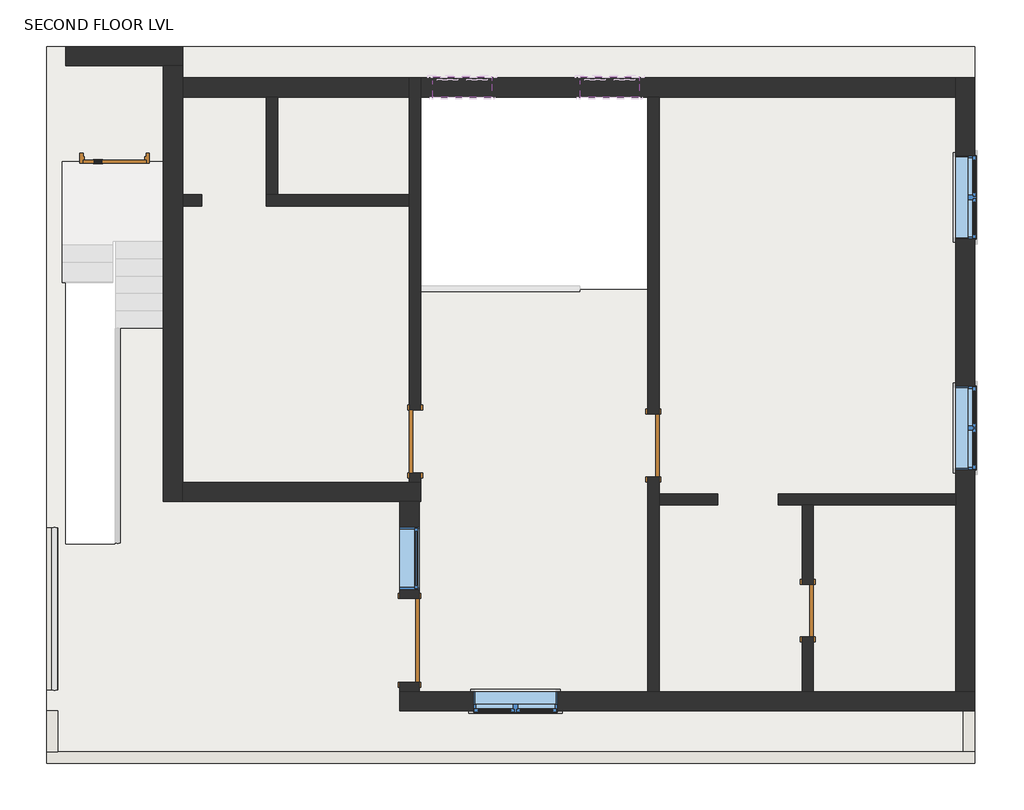
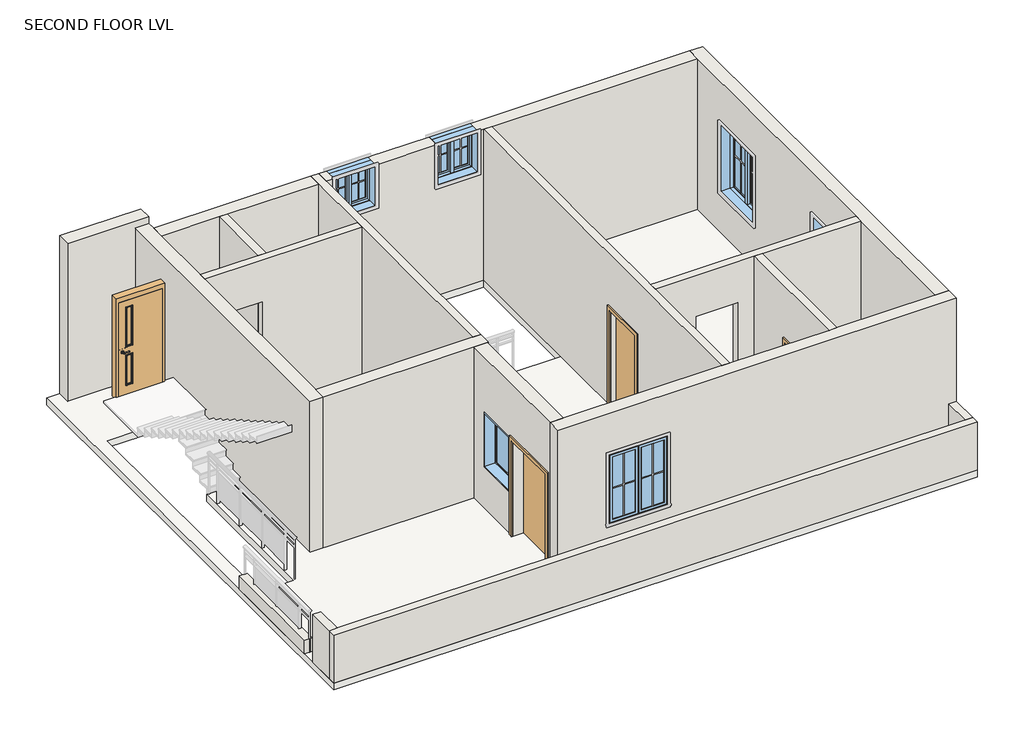
# One storey, part 1 of 2: 18 walls, 6 windows, 5 doors, 1 slab.
"""IFC4 building model written with IfcOpenShell, lengths in millimetres."""

from ifc_helpers import new_model, si_unit, frame, origin, place, context, project, spatial, polyline, outline, extrude, faceted_brep, transform, mapped, element, save
from components import door_52fb15b9, door_3dc6c820, door_d2d7de5b, door_44a3b16d, door_21b9160b, window_60f40170, window_6eb120d7, window_49c71971

model = new_model("IFC4")

# Units and contexts
model_context = context("Model", 3, world=origin())
ifc_project = project(units=[si_unit("LENGTHUNIT", "METRE", prefix="MILLI")], contexts=[model_context])

# Site, building, storey
site = spatial("IfcSite", under=ifc_project)
building = spatial("IfcBuilding", under=site)
storey = spatial("IfcBuildingStorey", under=building, Name="SECOND FLOOR LVL", Elevation=7010.4)

# Doors
placement = place(None, origin())
door_shape = door_52fb15b9(model_context)
element("IfcDoor", 1, ObjectType="Door-Passage-Single-Vision_Two_Lite : 36\" x 84\"", at=placement, inside=storey, context=model_context, shape_type="MappedRepresentation", body=[
    mapped(door_shape, transform((-6092.5155596, 7334.5576853, 7835.9), x_axis=(1.0, 0.0, 0.0), y_axis=(0.0, 1.0, 0.0), z_axis=(0.0, 0.0, 1.0))),
])
door_2_shape = door_3dc6c820(model_context)
element("IfcDoor", 2, ObjectType="Single-Flush : 30\" x 84\"", at=placement, inside=storey, context=model_context, shape_type="MappedRepresentation", body=[
    mapped(door_2_shape, transform((3997.6344404, 698.8076853, 7010.4), x_axis=(0.0, 1.0, 0.0), y_axis=(-1.0, 0.0, 0.0), z_axis=(0.0, 0.0, 1.0))),
])
door_3_shape = door_d2d7de5b(model_context)
element("IfcDoor", 3, ObjectType="Single-Flush : 36\" x 84\"", at=placement, inside=storey, context=model_context, shape_type="MappedRepresentation", body=[
    mapped(door_3_shape, transform((1749.7344404, 3105.4576853, 7010.4), x_axis=(0.0, -1.0, 0.0), y_axis=(1.0, 0.0, 0.0), z_axis=(0.0, 0.0, 1.0))),
])
door_4_shape = door_44a3b16d(model_context)
element("IfcDoor", 4, ObjectType="Single-Flush : 36\" x 84\"", at=placement, inside=storey, context=model_context, shape_type="MappedRepresentation", body=[
    mapped(door_4_shape, transform((-1717.3655596, 3162.6076853, 7010.4), x_axis=(0.0, -1.0, 0.0), y_axis=(1.0, 0.0, 0.0), z_axis=(0.0, 0.0, 1.0))),
])
door_5_shape = door_21b9160b(model_context)
element("IfcDoor", 5, ObjectType="Single-Flush : 48\" x 84\"", at=placement, inside=storey, context=model_context, shape_type="MappedRepresentation", body=[
    mapped(door_5_shape, transform((-1799.9155596, 267.0076853, 7010.4), x_axis=(0.0, -1.0, 0.0), y_axis=(1.0, 0.0, 0.0), z_axis=(0.0, 0.0, 1.0))),
])

# Slab
element("IfcSlab", 6, ObjectType="Generic - 6\"", at=placement, inside=storey, context=model_context, shape_type="SweptSolid", body=[
    extrude(outline(polyline([(6429.6844404, 8915.7076853), (6429.6844404, -1523.6923147), (-7083.1155596, -1523.6923147), (-7083.1155596, 8915.7076853), (6429.6844404, 8915.7076853)]), holes=[polyline([(-6092.5155596, 1670.3576853), (-6092.5155596, 4813.6076853), (-5381.3155596, 4813.6076853), (-5381.3155596, 7188.5076853), (-6092.5155596, 7188.5076853), (-6803.7155596, 7188.5076853), (-6803.7155596, 1670.3576853), (-6092.5155596, 1670.3576853)]), polyline([(1667.1844404, 8179.1076853), (-1634.8155596, 8179.1076853), (-1634.8155596, 5385.1076853), (-555.3155596, 5385.1076853), (1667.1844404, 5385.1076853), (1667.1844404, 8179.1076853)])]), frame((0.0, 0.0, 6858.0), z_axis=(0.0, 0.0, 1.0), x_axis=(1.0, 0.0, 0.0)), (0.0, 0.0, 1.0), 152.4),
])

# Walls
element("IfcWall", 7, ObjectType="4", at=placement, inside=storey, context=model_context, shape_type="Brep", body=[
    faceted_brep([(-1799.9155596, 2705.4076853, 9144.0), (-1799.9155596, 2705.4076853, 7010.4), (-1799.9155596, 2565.7076853, 7010.4), (-1799.9155596, 2565.7076853, 10363.2), (-1799.9155596, 5181.9076853, 10363.2), (-1799.9155596, 5410.5076853, 10363.2), (-1799.9155596, 6591.6076853, 10363.2), (-1799.9155596, 6756.7076853, 10363.2), (-1799.9155596, 8179.1076853, 10363.2), (-1799.9155596, 8458.5076853, 10363.2), (-1799.9155596, 8458.5076853, 7010.4), (-1799.9155596, 8179.1076853, 7010.4), (-1799.9155596, 6756.7076853, 7010.4), (-1799.9155596, 6591.6076853, 7010.4), (-1799.9155596, 3619.8076853, 7010.4), (-1799.9155596, 3619.8076853, 9144.0), (-1634.8155596, 2565.7076853, 7010.4), (-1634.8155596, 2705.4076853, 7010.4), (-1634.8155596, 2705.4076853, 9144.0), (-1634.8155596, 3619.8076853, 9144.0), (-1634.8155596, 3619.8076853, 7010.4), (-1634.8155596, 8179.1076853, 7010.4), (-1634.8155596, 8458.5076853, 7010.4), (-1634.8155596, 8458.5076853, 10363.2), (-1634.8155596, 8179.1076853, 10363.2), (-1634.8155596, 2565.7076853, 10363.2)], [[[0, 1, 2, 3, 4, 5, 6, 7, 8, 9, 10, 11, 12, 13, 14, 15]], [[16, 17, 18, 19, 20, 21, 22, 23, 24, 25]], [[2, 1, 17, 16]], [[14, 13, 12, 11, 10, 22, 21, 20]], [[9, 8, 7, 6, 5, 4, 3, 25, 24, 23]], [[3, 2, 16, 25]], [[18, 17, 1, 0]], [[19, 18, 0, 15]], [[20, 19, 15, 14]], [[10, 9, 23, 22]]]),
])
element("IfcWall", 8, ObjectType="4", at=placement, inside=storey, context=model_context, shape_type="Brep", body=[
    faceted_brep([(1667.1844404, 2648.2576853, 9144.0), (1667.1844404, 2648.2576853, 7010.4), (1667.1844404, -482.2923147, 7010.4), (1667.1844404, -482.2923147, 10363.2), (1667.1844404, 8179.1076853, 10363.2), (1667.1844404, 8179.1076853, 7010.4), (1667.1844404, 3562.6576853, 7010.4), (1667.1844404, 3562.6576853, 9144.0), (1832.2844404, -482.2923147, 7010.4), (1832.2844404, 2235.5076853, 7010.4), (1832.2844404, 2400.6076853, 7010.4), (1832.2844404, 2648.2576853, 7010.4), (1832.2844404, 2648.2576853, 9144.0), (1832.2844404, 3562.6576853, 9144.0), (1832.2844404, 3562.6576853, 7010.4), (1832.2844404, 8179.1076853, 7010.4), (1832.2844404, 8179.1076853, 10363.2), (1832.2844404, 5410.5076853, 10363.2), (1832.2844404, 5181.9076853, 10363.2), (1832.2844404, 2514.9076853, 10363.2), (1832.2844404, 2400.6076853, 10363.2), (1832.2844404, 2235.5076853, 10363.2), (1832.2844404, -482.2923147, 10363.2)], [[[0, 1, 2, 3, 4, 5, 6, 7]], [[8, 9, 10, 11, 12, 13, 14, 15, 16, 17, 18, 19, 20, 21, 22]], [[6, 5, 15, 14]], [[2, 1, 11, 10, 9, 8]], [[4, 3, 22, 21, 20, 19, 18, 17, 16]], [[3, 2, 8, 22]], [[5, 4, 16, 15]], [[12, 11, 1, 0]], [[13, 12, 0, 7]], [[14, 13, 7, 6]]]),
])
element("IfcWall", 9, ObjectType="4", at=placement, inside=storey, context=model_context, shape_type="SweptSolid", body=[
    extrude(outline(polyline([(2235.5076853, 7010.4), (1079.8076853, 7010.4), (1079.8076853, 9144.0), (317.8076853, 9144.0), (317.8076853, 7010.4), (-482.2923147, 7010.4), (-482.2923147, 10363.2), (2235.5076853, 10363.2), (2235.5076853, 7010.4)])), frame((3915.0844404, 0.0, 0.0), z_axis=(1.0, 0.0, 0.0), x_axis=(0.0, 1.0, 0.0)), (0.0, 0.0, 1.0), 165.1),
])
element("IfcWall", 10, ObjectType="4", at=placement, inside=storey, context=model_context, shape_type="Brep", body=[
    faceted_brep([(6150.2844404, 2235.5076853, 7010.4), (6150.2844404, 2235.5076853, 10363.2), (4080.1844404, 2235.5076853, 10363.2), (3915.0844404, 2235.5076853, 10363.2), (1832.2844404, 2235.5076853, 10363.2), (1832.2844404, 2235.5076853, 7010.4), (2687.0502939, 2235.5076853, 7010.4), (2687.0502939, 2235.5076853, 9448.8), (3567.6284806, 2235.5076853, 9448.8), (3567.6284806, 2235.5076853, 7010.4), (3915.0844404, 2235.5076853, 7010.4), (4080.1844404, 2235.5076853, 7010.4), (6150.2844404, 2400.6076853, 10363.2), (6150.2844404, 2400.6076853, 7010.4), (3567.6284806, 2400.6076853, 7010.4), (3567.6284806, 2400.6076853, 9448.8), (2687.0502939, 2400.6076853, 9448.8), (2687.0502939, 2400.6076853, 7010.4), (1832.2844404, 2400.6076853, 7010.4), (1832.2844404, 2400.6076853, 10363.2), (2022.7844404, 2400.6076853, 10363.2), (5307.0165832, 2400.6076853, 10363.2), (5611.8165832, 2400.6076853, 10363.2)], [[[0, 1, 2, 3, 4, 5, 6, 7, 8, 9, 10, 11]], [[12, 13, 14, 15, 16, 17, 18, 19, 20, 21, 22]], [[5, 18, 17, 6]], [[13, 0, 11, 10, 9, 14]], [[4, 3, 2, 1, 12, 22, 21, 20, 19]], [[1, 0, 13, 12]], [[5, 4, 19, 18]], [[7, 16, 15, 8]], [[16, 7, 6, 17]], [[8, 15, 14, 9]]]),
])
element("IfcWall", 11, ObjectType="4", at=placement, inside=storey, context=model_context, shape_type="SweptSolid", body=[
    extrude(outline(polyline([(-3882.7155596, 6756.7076853), (-3882.7155596, 8179.1076853), (-3717.6155596, 8179.1076853), (-3717.6155596, 6756.7076853), (-3882.7155596, 6756.7076853)])), frame((0.0, 0.0, 7010.4), z_axis=(0.0, 0.0, 1.0), x_axis=(1.0, 0.0, 0.0)), (0.0, 0.0, 1.0), 3352.8),
])
element("IfcWall", 12, ObjectType="4", at=placement, inside=storey, context=model_context, shape_type="Brep", body=[
    faceted_brep([(-1799.9155596, 6591.6076853, 7010.4), (-1799.9155596, 6591.6076853, 10363.2), (-5101.9155596, 6591.6076853, 10363.2), (-5101.9155596, 6591.6076853, 7010.4), (-4820.8679217, 6591.6076853, 7010.4), (-4820.8679217, 6591.6076853, 9448.8), (-3885.4711324, 6591.6076853, 9448.8), (-3885.4711324, 6591.6076853, 7010.4), (-1799.9155596, 6756.7076853, 10363.2), (-1799.9155596, 6756.7076853, 7010.4), (-3717.6155596, 6756.7076853, 7010.4), (-3882.7155596, 6756.7076853, 7010.4), (-3885.4711324, 6756.7076853, 7010.4), (-3885.4711324, 6756.7076853, 9448.8), (-4820.8679217, 6756.7076853, 9448.8), (-4820.8679217, 6756.7076853, 7010.4), (-5101.9155596, 6756.7076853, 7010.4), (-5101.9155596, 6756.7076853, 10363.2), (-3882.7155596, 6756.7076853, 10363.2), (-3717.6155596, 6756.7076853, 10363.2)], [[[0, 1, 2, 3, 4, 5, 6, 7]], [[8, 9, 10, 11, 12, 13, 14, 15, 16, 17, 18, 19]], [[9, 0, 7, 12, 11, 10]], [[3, 16, 15, 4]], [[2, 1, 8, 19, 18, 17]], [[1, 0, 9, 8]], [[3, 2, 17, 16]], [[5, 14, 13, 6]], [[14, 5, 4, 15]], [[6, 13, 12, 7]]]),
])
element("IfcWall", 13, ObjectType="4", at=placement, inside=storey, context=model_context, shape_type="SweptSolid", body=[
    extrude(outline(polyline([(-6918.0155596, 1905.3076853), (-6918.0155596, -456.8923147), (-7083.1155596, -456.8923147), (-7083.1155596, 1905.3076853), (-6918.0155596, 1905.3076853)])), frame((0.0, 0.0, 7010.4), z_axis=(0.0, 0.0, 1.0), x_axis=(1.0, 0.0, 0.0)), (0.0, 0.0, 1.0), 304.8),
])
element("IfcWall", 14, ObjectType="4", at=placement, inside=storey, context=model_context, shape_type="Brep", body=[
    faceted_brep([(6429.6844404, -1358.5923147, 7010.4), (6264.5844404, -1358.5923147, 7010.4), (-6918.0155596, -1358.5923147, 7010.4), (-7083.1155596, -1358.5923147, 7010.4), (-7083.1155596, -1358.5923147, 8077.2), (-6918.0155596, -1358.5923147, 8077.2), (6264.5844404, -1358.5923147, 8077.2), (6429.6844404, -1358.5923147, 8077.2), (6429.6844404, -1523.6923147, 7010.4), (6429.6844404, -1523.6923147, 8077.2), (-7083.1155596, -1523.6923147, 8077.2), (-7083.1155596, -1523.6923147, 7010.4)], [[[0, 1, 2, 3, 4, 5, 6, 7]], [[8, 9, 10, 11]], [[3, 2, 1, 0, 8, 11]], [[7, 6, 5, 4, 10, 9]], [[4, 3, 11, 10]], [[0, 7, 9, 8]]]),
])
element("IfcWall", 15, ObjectType="4", at=placement, inside=storey, context=model_context, shape_type="SweptSolid", body=[
    extrude(outline(polyline([(-6918.0155596, -761.6923147), (-6918.0155596, -1358.5923147), (-7083.1155596, -1358.5923147), (-7083.1155596, -761.6923147), (-6918.0155596, -761.6923147)])), frame((0.0, 0.0, 7010.4), z_axis=(0.0, 0.0, 1.0), x_axis=(1.0, 0.0, 0.0)), (0.0, 0.0, 1.0), 1066.8),
])
element("IfcWall", 16, ObjectType="4", at=placement, inside=storey, context=model_context, shape_type="SweptSolid", body=[
    extrude(outline(polyline([(6429.6844404, -761.6923147), (6429.6844404, -1358.5923147), (6264.5844404, -1358.5923147), (6264.5844404, -761.6923147), (6429.6844404, -761.6923147)])), frame((0.0, 0.0, 7010.4), z_axis=(0.0, 0.0, 1.0), x_axis=(1.0, 0.0, 0.0)), (0.0, 0.0, 1.0), 1066.8),
])
element("IfcWall", 17, ObjectType="9", at=placement, inside=storey, context=model_context, shape_type="Brep", body=[
    faceted_brep([(-1939.6155596, -761.6923147, 7010.4), (6264.5844404, -761.6923147, 7010.4), (6429.6844404, -761.6923147, 7010.4), (6429.6844404, -761.6923147, 8077.2), (6429.6844404, -761.6923147, 10363.2), (-1939.6155596, -761.6923147, 10363.2), (-866.4655596, -761.6923147, 9448.8), (352.7344404, -761.6923147, 9448.8), (352.7344404, -761.6923147, 7924.8), (-866.4655596, -761.6923147, 7924.8), (-1939.6155596, -482.2923147, 7010.4), (-1939.6155596, -482.2923147, 10363.2), (-1660.2155596, -482.2923147, 10363.2), (1667.1844404, -482.2923147, 10363.2), (1832.2844404, -482.2923147, 10363.2), (3915.0844404, -482.2923147, 10363.2), (4080.1844404, -482.2923147, 10363.2), (6150.2844404, -482.2923147, 10363.2), (6429.6844404, -482.2923147, 10363.2), (6429.6844404, -482.2923147, 7010.4), (6150.2844404, -482.2923147, 7010.4), (4080.1844404, -482.2923147, 7010.4), (3915.0844404, -482.2923147, 7010.4), (1832.2844404, -482.2923147, 7010.4), (1667.1844404, -482.2923147, 7010.4), (-1660.2155596, -482.2923147, 7010.4), (-866.4655596, -482.2923147, 9448.8), (-866.4655596, -482.2923147, 7924.8), (352.7344404, -482.2923147, 7924.8), (352.7344404, -482.2923147, 9448.8)], [[[0, 1, 2, 3, 4, 5], [6, 7, 8, 9]], [[10, 11, 12, 13, 14, 15, 16, 17, 18, 19, 20, 21, 22, 23, 24, 25], [26, 27, 28, 29]], [[2, 1, 0, 10, 25, 24, 23, 22, 21, 20, 19]], [[5, 4, 18, 17, 16, 15, 14, 13, 12, 11]], [[27, 26, 6, 9]], [[28, 27, 9, 8]], [[29, 28, 8, 7]], [[26, 29, 7, 6]], [[0, 5, 11, 10]], [[2, 19, 18, 4, 3]]]),
])
element("IfcWall", 18, ObjectType="9", at=placement, inside=storey, context=model_context, shape_type="Brep", body=[
    faceted_brep([(6429.6844404, -482.2923147, 10363.2), (6429.6844404, -482.2923147, 7010.4), (6429.6844404, 8458.5076853, 7010.4), (6429.6844404, 8458.5076853, 10363.2), (6429.6844404, 2749.8576853, 9448.8), (6429.6844404, 3969.0576853, 9448.8), (6429.6844404, 3969.0576853, 7924.8), (6429.6844404, 2749.8576853, 7924.8), (6429.6844404, 6109.0076853, 9448.8), (6429.6844404, 7328.2076853, 9448.8), (6429.6844404, 7328.2076853, 7924.8), (6429.6844404, 6109.0076853, 7924.8), (6150.2844404, -482.2923147, 7010.4), (6150.2844404, -482.2923147, 10363.2), (6150.2844404, 2235.5076853, 10363.2), (6150.2844404, 2400.6076853, 10363.2), (6150.2844404, 8179.1076853, 10363.2), (6150.2844404, 8458.5076853, 10363.2), (6150.2844404, 8458.5076853, 7010.4), (6150.2844404, 8179.1076853, 7010.4), (6150.2844404, 2400.6076853, 7010.4), (6150.2844404, 2235.5076853, 7010.4), (6150.2844404, 2749.8576853, 9448.8), (6150.2844404, 2749.8576853, 7924.8), (6150.2844404, 3969.0576853, 7924.8), (6150.2844404, 3969.0576853, 9448.8), (6150.2844404, 6109.0076853, 9448.8), (6150.2844404, 6109.0076853, 7924.8), (6150.2844404, 7328.2076853, 7924.8), (6150.2844404, 7328.2076853, 9448.8)], [[[0, 1, 2, 3], [4, 5, 6, 7], [8, 9, 10, 11]], [[12, 13, 14, 15, 16, 17, 18, 19, 20, 21], [22, 23, 24, 25], [26, 27, 28, 29]], [[2, 1, 12, 21, 20, 19, 18]], [[0, 3, 17, 16, 15, 14, 13]], [[3, 2, 18, 17]], [[23, 22, 4, 7]], [[24, 23, 7, 6]], [[25, 24, 6, 5]], [[22, 25, 5, 4]], [[27, 26, 8, 11]], [[28, 27, 11, 10]], [[29, 28, 10, 9]], [[26, 29, 9, 8]], [[0, 13, 12, 1]]]),
])
element("IfcWall", 19, ObjectType="9", at=placement, inside=storey, context=model_context, shape_type="Brep", body=[
    faceted_brep([(6150.2844404, 8458.5076853, 7010.4), (-1634.8155596, 8458.5076853, 7010.4), (-1634.8155596, 8458.5076853, 10363.2), (-1463.3655596, 8458.5076853, 10363.2), (-1463.3655596, 8458.5076853, 9448.8), (-599.7655596, 8458.5076853, 9448.8), (-599.7655596, 8458.5076853, 10363.2), (682.9344404, 8458.5076853, 10363.2), (682.9344404, 8458.5076853, 9448.8), (1546.5344404, 8458.5076853, 9448.8), (1546.5344404, 8458.5076853, 10363.2), (6150.2844404, 8458.5076853, 10363.2), (-1634.8155596, 8179.1076853, 7010.4), (1667.1844404, 8179.1076853, 7010.4), (1832.2844404, 8179.1076853, 7010.4), (6150.2844404, 8179.1076853, 7010.4), (6150.2844404, 8179.1076853, 10363.2), (1832.2844404, 8179.1076853, 10363.2), (1667.1844404, 8179.1076853, 10363.2), (1546.5344404, 8179.1076853, 10363.2), (1546.5344404, 8179.1076853, 9448.8), (682.9344404, 8179.1076853, 9448.8), (682.9344404, 8179.1076853, 10363.2), (-599.7655596, 8179.1076853, 10363.2), (-599.7655596, 8179.1076853, 9448.8), (-1463.3655596, 8179.1076853, 9448.8), (-1463.3655596, 8179.1076853, 10363.2), (-1634.8155596, 8179.1076853, 10363.2)], [[[0, 1, 2, 3, 4, 5, 6, 7, 8, 9, 10, 11]], [[12, 13, 14, 15, 16, 17, 18, 19, 20, 21, 22, 23, 24, 25, 26, 27]], [[1, 0, 15, 14, 13, 12]], [[16, 11, 10, 19, 18, 17]], [[2, 27, 26, 3]], [[22, 7, 6, 23]], [[0, 11, 16, 15]], [[2, 1, 12, 27]], [[9, 20, 19, 10]], [[20, 9, 8, 21]], [[21, 8, 7, 22]], [[5, 24, 23, 6]], [[24, 5, 4, 25]], [[25, 4, 3, 26]]]),
])
element("IfcWall", 20, ObjectType="9", at=placement, inside=storey, context=model_context, shape_type="Brep", body=[
    faceted_brep([(-6803.7155596, 8636.3076853, 7010.4), (-5381.3155596, 8636.3076853, 7010.4), (-5101.9155596, 8636.3076853, 7010.4), (-5101.9155596, 8636.3076853, 10363.2), (-5101.9155596, 8636.3076853, 10515.6), (-6803.7155596, 8636.3076853, 10515.6), (-6803.7155596, 8915.7076853, 7010.4), (-6803.7155596, 8915.7076853, 10515.6), (-5101.9155596, 8915.7076853, 10515.6), (-5101.9155596, 8915.7076853, 7010.4)], [[[0, 1, 2, 3, 4, 5]], [[6, 7, 8, 9]], [[2, 1, 0, 6, 9]], [[5, 4, 8, 7]], [[0, 5, 7, 6]], [[4, 3, 2, 9, 8]]]),
])
element("IfcWall", 21, ObjectType="9", at=placement, inside=storey, context=model_context, shape_type="Brep", body=[
    faceted_brep([(-5381.3155596, 8636.3076853, 7010.4), (-5381.3155596, 2286.3076853, 7010.4), (-5381.3155596, 2286.3076853, 10363.2), (-5381.3155596, 8636.3076853, 10363.2), (-5101.9155596, 8636.3076853, 7010.4), (-5101.9155596, 8636.3076853, 10363.2), (-5101.9155596, 8458.5076853, 10363.2), (-5101.9155596, 8179.1076853, 10363.2), (-5101.9155596, 6756.7076853, 10363.2), (-5101.9155596, 6591.6076853, 10363.2), (-5101.9155596, 2565.7076853, 10363.2), (-5101.9155596, 2286.3076853, 10363.2), (-5101.9155596, 2286.3076853, 7010.4), (-5101.9155596, 2565.7076853, 7010.4), (-5101.9155596, 2591.1076853, 7010.4), (-5101.9155596, 6591.6076853, 7010.4), (-5101.9155596, 6756.7076853, 7010.4), (-5101.9155596, 8179.1076853, 7010.4), (-5101.9155596, 8458.5076853, 7010.4), (-5330.5155596, 2286.3076853, 7010.4)], [[[0, 1, 2, 3]], [[4, 5, 6, 7, 8, 9, 10, 11, 12, 13, 14, 15, 16, 17, 18]], [[1, 0, 4, 18, 17, 16, 15, 14, 13, 12, 19]], [[3, 2, 11, 10, 9, 8, 7, 6, 5]], [[0, 3, 5, 4]], [[2, 1, 19, 12, 11]]]),
])
element("IfcWall", 22, ObjectType="9", at=placement, inside=storey, context=model_context, shape_type="Brep", body=[
    faceted_brep([(-5101.9155596, 2286.3076853, 7010.4), (-1939.6155596, 2286.3076853, 7010.4), (-1660.2155596, 2286.3076853, 7010.4), (-1634.8155596, 2286.3076853, 7010.4), (-1634.8155596, 2286.3076853, 10363.2), (-1660.2155596, 2286.3076853, 10363.2), (-1939.6155596, 2286.3076853, 10363.2), (-5101.9155596, 2286.3076853, 10363.2), (-5101.9155596, 2565.7076853, 7010.4), (-5101.9155596, 2565.7076853, 10363.2), (-1799.9155596, 2565.7076853, 10363.2), (-1634.8155596, 2565.7076853, 10363.2), (-1634.8155596, 2565.7076853, 7010.4), (-1799.9155596, 2565.7076853, 7010.4), (-1634.8155596, 2514.9076853, 7010.4)], [[[0, 1, 2, 3, 4, 5, 6, 7]], [[8, 9, 10, 11, 12, 13]], [[3, 2, 1, 0, 8, 13, 12, 14]], [[7, 6, 5, 4, 11, 10, 9]], [[0, 7, 9, 8]], [[4, 3, 14, 12, 11]]]),
])
element("IfcWall", 23, ObjectType="9", at=placement, inside=storey, context=model_context, shape_type="SweptSolid", body=[
    extrude(outline(polyline([(-342.5923147, 9144.0), (-342.5923147, 7010.4), (-482.2923147, 7010.4), (-482.2923147, 10363.2), (2286.3076853, 10363.2), (2286.3076853, 7010.4), (876.6076853, 7010.4), (876.6076853, 9144.0), (-342.5923147, 9144.0)]), holes=[polyline([(1003.6076853, 9144.0), (1003.6076853, 7924.8), (1918.0076853, 7924.8), (1918.0076853, 9144.0), (1003.6076853, 9144.0)])]), frame((-1939.6155596, 0.0, 0.0), z_axis=(1.0, 0.0, 0.0), x_axis=(0.0, 1.0, 0.0)), (0.0, 0.0, 1.0), 279.4),
])
element("IfcWall", 24, ObjectType="9", at=placement, inside=storey, context=model_context, shape_type="Brep", body=[
    faceted_brep([(-5101.9155596, 8179.1076853, 7010.4), (-3882.7155596, 8179.1076853, 7010.4), (-3717.6155596, 8179.1076853, 7010.4), (-1799.9155596, 8179.1076853, 7010.4), (-1799.9155596, 8179.1076853, 10363.2), (-3717.6155596, 8179.1076853, 10363.2), (-3882.7155596, 8179.1076853, 10363.2), (-5101.9155596, 8179.1076853, 10363.2), (-5101.9155596, 8458.5076853, 7010.4), (-5101.9155596, 8458.5076853, 10363.2), (-1799.9155596, 8458.5076853, 10363.2), (-1799.9155596, 8458.5076853, 7010.4), (-1939.6155596, 8458.5076853, 7010.4), (-5025.7155596, 8458.5076853, 7010.4), (-5101.9155596, 8229.9076853, 7010.4), (-1799.9155596, 8229.9076853, 7010.4)], [[[0, 1, 2, 3, 4, 5, 6, 7]], [[8, 9, 10, 11, 12, 13]], [[3, 2, 1, 0, 14, 8, 13, 12, 11, 15]], [[7, 6, 5, 4, 10, 9]], [[4, 3, 15, 11, 10]], [[0, 7, 9, 8, 14]]]),
])

# Windows
window_shape = window_60f40170(model_context)
element("IfcWindow", 25, ObjectType="Fixed : 36\" x 48\"", at=placement, inside=storey, context=model_context, shape_type="MappedRepresentation", body=[
    mapped(window_shape, transform((-1799.9155596, 1422.7076853, 7010.4), x_axis=(0.0, -1.0, 0.0), y_axis=(1.0, 0.0, 0.0), z_axis=(0.0, 0.0, 1.0))),
])
window_2_shape = window_6eb120d7(model_context)
element("IfcWindow", 26, ObjectType="Window-Casement-Double : 34\" x 36\"", at=placement, inside=storey, context=model_context, shape_type="MappedRepresentation", body=[
    mapped(window_2_shape, transform((-1031.5655596, 8318.8076853, 8534.4), x_axis=(1.0, 0.0, 0.0), y_axis=(0.0, 1.0, 0.0), z_axis=(0.0, 0.0, 1.0))),
])
element("IfcWindow", 27, ObjectType="Window-Casement-Double : 34\" x 36\"", at=placement, inside=storey, context=model_context, shape_type="MappedRepresentation", body=[
    mapped(window_2_shape, transform((1114.7344404, 8318.8076853, 8534.4), x_axis=(1.0, 0.0, 0.0), y_axis=(0.0, 1.0, 0.0), z_axis=(0.0, 0.0, 1.0))),
])
window_3_shape = window_49c71971(model_context)
element("IfcWindow", 28, ObjectType="Window-Casement-Double : 48\" x 60\"", at=placement, inside=storey, context=model_context, shape_type="MappedRepresentation", body=[
    mapped(window_3_shape, transform((-256.8655596, -621.9923147, 7010.4), x_axis=(-1.0, 0.0, 0.0), y_axis=(0.0, -1.0, 0.0), z_axis=(0.0, 0.0, 1.0))),
])
element("IfcWindow", 29, ObjectType="Window-Casement-Double : 48\" x 60\"", at=placement, inside=storey, context=model_context, shape_type="MappedRepresentation", body=[
    mapped(window_3_shape, transform((6289.9844404, 3359.4576853, 7010.4), x_axis=(0.0, -1.0, 0.0), y_axis=(1.0, 0.0, 0.0), z_axis=(0.0, 0.0, 1.0))),
])
element("IfcWindow", 30, ObjectType="Window-Casement-Double : 48\" x 60\"", at=placement, inside=storey, context=model_context, shape_type="MappedRepresentation", body=[
    mapped(window_3_shape, transform((6289.9844404, 6718.6076853, 7010.4), x_axis=(0.0, -1.0, 0.0), y_axis=(1.0, 0.0, 0.0), z_axis=(0.0, 0.0, 1.0))),
])

save(model, "model.ifc")

# Revit data of these elements
# Type "Door-Passage-Single-Vision_Two_Lite : 36\" x 84\""
#   Type Mark = "9"
#   Assembly Code = "B2030100"
#   Analytic Construction = "Wooden"
#   Thickness = 0' - 1 3/4"
#   Thermal Resistance (R) = 2.5876 (h·ft²·°F)/BTU
#   Swing Angle [instance default] = 90.00°
#   Strike Height = 3' - 4"
#   Rough Width [instance default] = 3' - 4"
#   Rough Height [instance default] = 7' - 4"
#   MF Opening Height [instance default] = 0' - 4"
#   MF Opening Width [instance default] = 0' - 4"
#   Heat Transfer Coefficient (U) = 0.3865 BTU/(h·ft²·°F)
#   Inset Calculate [instance default] = 0' - 4"
#   Masonry Inset [instance default] = 0' - 1"
#   Height = 7' - 0"
#   Width = 3' - 0"
#   Masonry Frame Depth = 0' - 5 3/4"
#   Masonry Frame [instance default] = yes
#   Function = 1
#   Dry Wall Frame [instance default] = no
#   Panel Material = Wood - Birch
#   Glazing = Glass
#   Glass Stop Material = Metal - Paint Finish - Grey
#   Frame Material = Metal - Paint Finish - Grey
#   Door Handle Material = Aluminum
#   Visual Light Transmittance = 0
#   Solar Heat Gain Coefficient = 0
#   Wall Closure = (empty or 0)
# Type "Single-Flush : 30\" x 84\""
#   Type Mark = "4"
#   Construction Type Id = "MDOOR"
#   Assembly Code = "C1020"
#   Analytic Construction = "Metal"
#   Thickness = 0' - 2"
#   Heat Transfer Coefficient (U) = 0.651978 BTU/(h·ft²·°F)
#   Height = 7' - 0"
#   Trim Projection Ext = 0' - 1"
#   Trim Projection Int = 0' - 1"
#   Trim Width = 0' - 3"
#   Width = 2' - 6"
#   Define Thermal Properties by = 1
#   Define Thermal Properties by = 1
#   Door Material = Door - Panel
#   Frame Material = Door - Frame
#   Visual Light Transmittance = 0
#   Solar Heat Gain Coefficient = 0
#   Function = (empty or 0)
#   Wall Closure = (empty or 0)
# Type "Single-Flush : 36\" x 84\""
#   Type Mark = "1"
#   Construction Type Id = "MDOOR"
#   Assembly Code = "C1020"
#   Analytic Construction = "Metal"
#   Thickness = 0' - 2"
#   Heat Transfer Coefficient (U) = 0.651978 BTU/(h·ft²·°F)
#   Height = 7' - 0"
#   Trim Projection Ext = 0' - 1"
#   Trim Projection Int = 0' - 1"
#   Trim Width = 0' - 3"
#   Width = 3' - 0"
#   Define Thermal Properties by = 1
#   Define Thermal Properties by = 1
#   Door Material = Door - Panel
#   Frame Material = Door - Frame
#   Visual Light Transmittance = 0
#   Solar Heat Gain Coefficient = 0
#   Function = (empty or 0)
#   Wall Closure = (empty or 0)
# Type "Single-Flush : 48\" x 84\""
#   Type Mark = "8"
#   Construction Type Id = "MDOOR"
#   Assembly Code = "C1020"
#   Analytic Construction = "Metal"
#   Thickness = 0' - 2"
#   Heat Transfer Coefficient (U) = 0.651978 BTU/(h·ft²·°F)
#   Height = 7' - 0"
#   Trim Projection Ext = 0' - 1"
#   Trim Projection Int = 0' - 1"
#   Trim Width = 0' - 3"
#   Width = 4' - 0"
#   Define Thermal Properties by = 1
#   Door Material = Door - Panel
#   Frame Material = Door - Frame
#   Visual Light Transmittance = 0
#   Solar Heat Gain Coefficient = 0
#   Function = (empty or 0)
#   Wall Closure = (empty or 0)
# Type "Generic - 6\""
#   Assembly Code = "B1010"
#   Function = 0
#   Layers, outside or top first: 0' - 6" no material (function 1)
# Type "4"
#   Assembly Code = "B2010"
#   Layers, outside or top first: 0' - 1" "Gypsum Wall Board" (function 1); 0' - 4 1/2" no material (function 1); 0' - 1" "Gypsum Wall Board" (function 1)
# Type "9"
#   Assembly Code = "B2010"
#   Layers, outside or top first: 0' - 1" "Gypsum Wall Board" (function 1); 0' - 9" no material (function 1); 0' - 1" "Gypsum Wall Board" (function 1)
# Type "Fixed : 36\" x 48\""
#   Type Mark = "1"
#   Construction Type Id = "GSP4R"
#   Assembly Code = "B2020100"
#   Analytic Construction = "1/8 in Pilkington single glazing"
#   Visual Light Transmittance = 0.9
#   Solar Heat Gain Coefficient = 0.78
#   Heat Transfer Coefficient (U) = 0.6496 BTU/(h·ft²·°F)
#   Height = 4' - 0"
#   Default Sill Height = 3' - 0"
#   Width = 3' - 0"
#   Window Inset = 0' - 0 3/4"
#   Define Thermal Properties by = 1
#   Define Thermal Properties by = 1
#   Glass Pane Material = Glass
#   Sash Material = Sash
#   Wall Closure = (empty or 0)
# Type "Window-Casement-Double : 34\" x 36\""
#   Type Mark = "14"
#   Fire Rating = "0.5h"
#   Assembly Code = "B2020100"
#   Analytic Construction = "Double glazing - domestic"
#   Frame Extension [instance default] = 0' - 0 1/4"
#   Window Inset [instance default] = 0' - 0"
#   Wall Thickness [instance default] = 0' - 6"
#   Interior Wall Closure [instance default] = 0' - 2 1/4"
#   Half Width = 1' - 5"
#   Visual Light Transmittance = 0.81
#   Thermal Resistance (R) = 1.8146 (h·ft²·°F)/BTU
#   Solar Heat Gain Coefficient = 0.76
#   Rough Width = 2' - 10 1/2"
#   Rough Height = 3' - 0 1/2"
#   Height = 3' - 0"
#   Heat Transfer Coefficient (U) = 0.5511 BTU/(h·ft²·°F)
#   Exterior Wall Closure [instance default] = 0' - 1 1/4"
#   Extension Jamb [instance default] = 0' - 2 1/4"
#   Default Sill Height = 3' - 0"
#   Width = 2' - 10"
#   Define Thermal Properties by = 0
#   Muntin Visibility = yes
#   Interior Trim Visibility [instance default] = yes
#   Exterior Trim Visibility [instance default] = yes
#   Extension Jamb Visibility [instance default] = yes
#   Interior Trim Material = Wood - Stained
#   Muntin Pattern = Muntin Pattern_2x2 : Muntin Pattern_2x2
#   Interior Trim = Trim-Window-Interior-Flat : Picture Frame
#   Interior Frame Material = Wood - Stained
#   Glass Panel Material = Glass
#   Exterior Trim Material = Clad - White
#   Exterior Trim = Trim-Window-Exterior-Flat : with Sill
#   Exterior Frame Material = Clad - White
#   Wall Closure = (empty or 0)
# Type "Window-Casement-Double : 48\" x 60\""
#   Type Mark = "16"
#   Fire Rating = "0.5h"
#   Assembly Code = "B2020100"
#   Analytic Construction = "Double glazing - domestic"
#   Frame Extension [instance default] = 0' - 0 1/4"
#   Window Inset [instance default] = 0' - 0"
#   Wall Thickness [instance default] = 0' - 6"
#   Interior Wall Closure [instance default] = 0' - 2 1/4"
#   Half Width = 2' - 0"
#   Visual Light Transmittance = 0.81
#   Thermal Resistance (R) = 1.8146 (h·ft²·°F)/BTU
#   Solar Heat Gain Coefficient = 0.76
#   Rough Width = 4' - 0 1/2"
#   Rough Height = 5' - 0 1/2"
#   Height = 5' - 0"
#   Heat Transfer Coefficient (U) = 0.5511 BTU/(h·ft²·°F)
#   Exterior Wall Closure [instance default] = 0' - 1 1/4"
#   Extension Jamb [instance default] = 0' - 2 1/4"
#   Default Sill Height = 3' - 0"
#   Width = 4' - 0"
#   Define Thermal Properties by = 0
#   Muntin Visibility = yes
#   Interior Trim Visibility [instance default] = yes
#   Exterior Trim Visibility [instance default] = yes
#   Extension Jamb Visibility [instance default] = yes
#   Interior Trim Material = Wood - Stained
#   Muntin Pattern = Muntin Pattern_2x2 : Muntin Pattern_2x2
#   Interior Trim = Trim-Window-Interior-Flat : Picture Frame
#   Interior Frame Material = Wood - Stained
#   Glass Panel Material = Glass
#   Exterior Trim Material = Clad - White
#   Exterior Trim = Trim-Window-Exterior-Flat : with Sill
#   Exterior Frame Material = Clad - White
#   Wall Closure = (empty or 0)
# Element 1 (IfcDoor, "Door-Passage-Single-Vision_Two_Lite : 36\" x 84\"")
#   Swing Angle = 90.00°
#   Rough Width = 3' - 4"
#   Rough Height = 7' - 4"
#   Masonry Inset = 0' - 1"
#   MF Opening Width = 0' - 4"
#   MF Opening Height = 0' - 4"
#   Inset Calculate = 0' - 4"
#   Masonry Frame = yes
#   Dry Wall Frame = no
#   Phase Created = New Construction
#   Materials on its faces: "Metal - Paint Finish - Grey", "Aluminum", "Wood - Birch", "Glass"
# Element 2 (IfcDoor, "Single-Flush : 30\" x 84\"")
#   Phase Created = New Construction
#   Materials on its faces: "Door - Frame", "Door - Panel"
# Elements 3, 4 (IfcDoor, "Single-Flush : 36\" x 84\"")
#   Phase Created = New Construction
#   Materials on its faces: "Door - Frame", "Door - Panel"
# Element 5 (IfcDoor, "Single-Flush : 48\" x 84\"")
#   Phase Created = New Construction
#   Materials on its faces: "Door - Frame", "Door - Panel"
# Element 6 (IfcSlab, "Generic - 6\"")
#   Height Offset From Level = 0' - 0"
#   Phase Created = New Construction
#   Materials on its faces: "Default Floor"
# Elements 7, 8, 9, 10, 11, 12 (IfcWall, "4")
#   Top Offset = -0' - 6"
#   Base Offset = 0' - 0"
#   wall height = 11' - 0"
#   Phase Created = New Construction
#   Base Constraint = SECOND FLOOR LVL
#   Top Constraint = ROOF LVL
#   Materials on its faces: "Default Wall", "Gypsum Wall Board"
# Element 13 (IfcWall, "4")
#   Top Offset = 0' - 0"
#   Base Offset = 0' - 0"
#   Unconnected Height = 1' - 0"
#   wall height = 1' - 0"
#   Phase Created = New Construction
#   Base Constraint = SECOND FLOOR LVL
#   Materials on its faces: "Default Wall", "Gypsum Wall Board"
# Element 14 (IfcWall, "4")
#   Top Offset = 0' - 0"
#   Base Offset = 0' - 0"
#   Unconnected Height = 3' - 6"
#   wall height = 3' - 6"
#   Phase Created = New Construction
#   Base Constraint = SECOND FLOOR LVL
#   Materials on its faces: "Gypsum Wall Board", "Default Wall"
# Elements 15, 16 (IfcWall, "4")
#   Top Offset = 0' - 0"
#   Base Offset = 0' - 0"
#   Unconnected Height = 3' - 6"
#   wall height = 3' - 6"
#   Phase Created = New Construction
#   Base Constraint = SECOND FLOOR LVL
#   Materials on its faces: "Default Wall", "Gypsum Wall Board"
# Elements 17, 18, 19, 23, 24 (IfcWall, "9")
#   Top Offset = -0' - 6"
#   Base Offset = 0' - 0"
#   wall height = 11' - 0"
#   Phase Created = New Construction
#   Base Constraint = SECOND FLOOR LVL
#   Top Constraint = ROOF LVL
#   Materials on its faces: "Default Wall", "Gypsum Wall Board"
# Element 20 (IfcWall, "9")
#   Top Offset = 0' - 0"
#   Base Offset = 0' - 0"
#   wall height = 11' - 6"
#   Phase Created = New Construction
#   Base Constraint = SECOND FLOOR LVL
#   Top Constraint = ROOF LVL
#   Materials on its faces: "Gypsum Wall Board", "Default Wall"
# Elements 21, 22 (IfcWall, "9")
#   Top Offset = -0' - 6"
#   Base Offset = 0' - 0"
#   wall height = 11' - 0"
#   Phase Created = New Construction
#   Base Constraint = SECOND FLOOR LVL
#   Top Constraint = ROOF LVL
#   Materials on its faces: "Gypsum Wall Board", "Default Wall"
# Element 25 (IfcWindow, "Fixed : 36\" x 48\"")
#   Mark = "15"
#   Phase Created = New Construction
#   Materials on its faces: "Sash", "Glass"
# Element 26 (IfcWindow, "Window-Casement-Double : 34\" x 36\"")
#   Mark = "11"
#   Window Inset = 0' - 0"
#   Interior Wall Closure = 0' - 2 1/4"
#   Frame Extension = 0' - 0 1/4"
#   Exterior Wall Closure = 0' - 1 1/4"
#   Interior Trim Visibility = yes
#   Exterior Trim Visibility = yes
#   Phase Created = New Construction
#   Materials on its faces: "Wood - Stained", "Glass", "Clad - White"
# Element 27 (IfcWindow, "Window-Casement-Double : 34\" x 36\"")
#   Mark = "12"
#   Window Inset = 0' - 0"
#   Interior Wall Closure = 0' - 2 1/4"
#   Frame Extension = 0' - 0 1/4"
#   Exterior Wall Closure = 0' - 1 1/4"
#   Interior Trim Visibility = yes
#   Exterior Trim Visibility = yes
#   Phase Created = New Construction
#   Materials on its faces: "Wood - Stained", "Glass", "Clad - White"
# Element 28 (IfcWindow, "Window-Casement-Double : 48\" x 60\"")
#   Mark = "8"
#   Window Inset = 0' - 0"
#   Interior Wall Closure = 0' - 2 1/4"
#   Frame Extension = 0' - 0 1/4"
#   Exterior Wall Closure = 0' - 1 1/4"
#   Interior Trim Visibility = yes
#   Exterior Trim Visibility = yes
#   Phase Created = New Construction
#   Materials on its faces: "Wood - Stained", "Glass", "Clad - White"
# Element 29 (IfcWindow, "Window-Casement-Double : 48\" x 60\"")
#   Mark = "9"
#   Window Inset = 0' - 0"
#   Interior Wall Closure = 0' - 2 1/4"
#   Frame Extension = 0' - 0 1/4"
#   Exterior Wall Closure = 0' - 1 1/4"
#   Interior Trim Visibility = yes
#   Exterior Trim Visibility = yes
#   Phase Created = New Construction
#   Materials on its faces: "Wood - Stained", "Glass", "Clad - White"
# Element 30 (IfcWindow, "Window-Casement-Double : 48\" x 60\"")
#   Mark = "10"
#   Window Inset = 0' - 0"
#   Interior Wall Closure = 0' - 2 1/4"
#   Frame Extension = 0' - 0 1/4"
#   Exterior Wall Closure = 0' - 1 1/4"
#   Interior Trim Visibility = yes
#   Exterior Trim Visibility = yes
#   Phase Created = New Construction
#   Materials on its faces: "Wood - Stained", "Glass", "Clad - White"
# Materials
#   "Wood - Birch": class "Wood", colour RGB 166 116 52, transparency 0, Cost = 0
#   "Glass": class "Glass", colour RGB 0 128 192, transparency 0.75, Description = "Soda Lime Glass", Cost = 0
#   "Metal - Paint Finish - Grey": class "Paint", colour RGB 104 104 104, transparency 0, Cost = 0
#   "Aluminum": class "Metal", colour RGB 247 247 247, transparency 0, Description = "Aluminum 6061", Cost = 0
#   "Door - Panel": class "Wood", colour RGB 210 159 95, transparency 0, Cost = 0
#   "Door - Frame": colour RGB 118 70 51, transparency 0, Cost = 0
#   "Gypsum Wall Board": class "Generic", colour RGB 228 228 228, transparency 0, Description = "Gypsum Wall Board", Cost = 0
#   "Sash": class "Wood", colour RGB 224 178 126, transparency 0, Cost = 0
#   "Wood - Stained": class "Wood", colour RGB 224 178 126, transparency 0, Cost = 0
#   "Clad - White": class "Wood", colour RGB 242 242 238, transparency 0, Cost = 0
#   "Default Floor": colour RGB 128 128 128, transparency 0, Cost = 0
#   "Default Wall": colour RGB 128 128 128, transparency 0, Cost = 0
